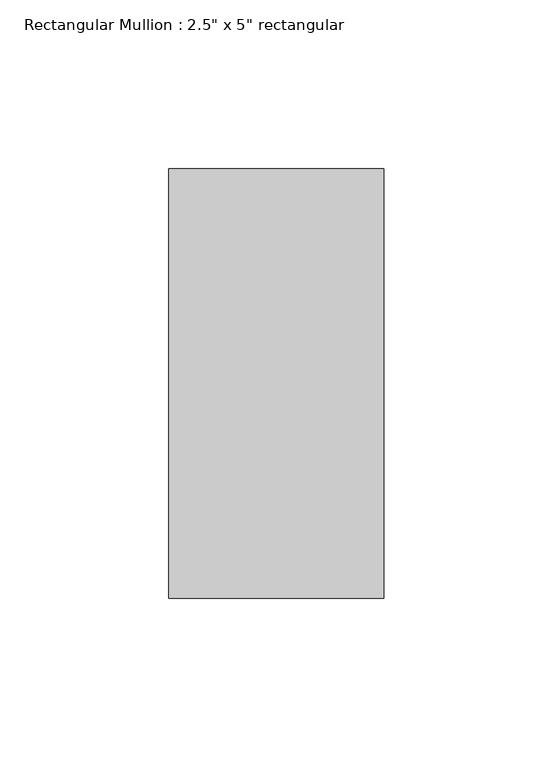
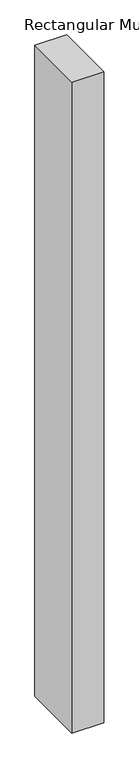
"""IFC4 building model written with IfcOpenShell, lengths in millimetres: member geometry."""

from ifc_helpers import new_model, si_unit, frame, origin, place, context, project, spatial, polyline, outline, extrude, source, transform, mapped, element, save


def member_22948727(model_context):
    return source(origin(), model_context, "Body", "SweptSolid", [
        extrude(outline(polyline([(0.0, 63.5), (0.0, -63.5), (-63.5, -63.5), (-63.5, 63.5), (0.0, 63.5)])), frame((0.0, 0.0, -1367.3666665), z_axis=(0.0, 0.0, 1.0), x_axis=(1.0, 0.0, 0.0)), (0.0, 0.0, 1.0), 1367.3666665),
    ])


if __name__ == "__main__":
    model = new_model("IFC4")
    model_context = context("Model", 3, world=origin())
    ifc_project = project(units=[si_unit("LENGTHUNIT", "METRE", prefix="MILLI")], contexts=[model_context])
    site = spatial("IfcSite", under=ifc_project)
    building = spatial("IfcBuilding", under=site)
    placement = place(None, origin())
    member_shape = member_22948727(model_context)
    element("IfcMember", 1, ObjectType="Rectangular Mullion : 2.5\" x 5\" rectangular", at=placement, inside=building, context=model_context, shape_type="MappedRepresentation", body=[
        mapped(member_shape, transform((0.0, 0.0, 0.0), x_axis=(1.0, 0.0, 0.0), y_axis=(0.0, 1.0, 0.0), z_axis=(0.0, 0.0, 1.0))),
    ])
    save(model, "model.ifc")

# Revit data of these elements
# Type "Rectangular Mullion : 2.5\" x 5\" rectangular"
#   built-in parameter 1007304 = 0.416667 (stored number, unit not read)
#   built-in parameter 1007301 = 0.104167 (stored number, unit not read)
#   built-in parameter 1007300 = 0.104167 (stored number, unit not read)
# Element 1 (IfcMember, "Rectangular Mullion : 2.5\" x 5\" rectangular")
#   Materials on its faces: "Aluminum"
# Materials
#   "Aluminum": class "Metal", colour RGB 247 247 247, transparency 0, Description = "Aluminum 6061", Cost = 0
